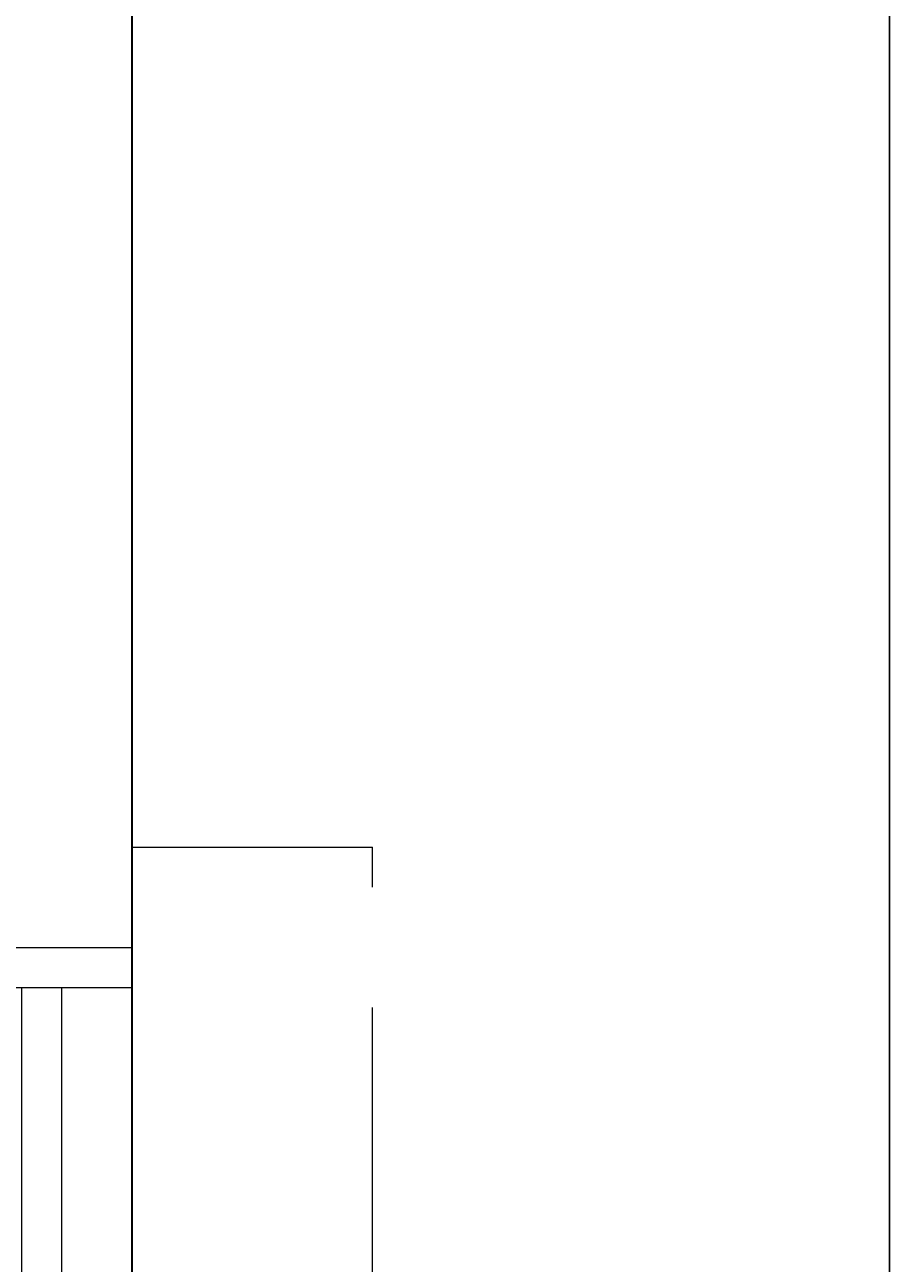
# Model space of a CAD drawing. Units: inches. Extents: x -128 to 854, y -395 to 398.
# Tile 32 of 61: x 309 to 352, y 2 to 64. Entities that reach past the tile are written whole.
import ezdxf

# ---------------------------------------------------------------- set-up
doc = ezdxf.new("R2010")
doc.units = ezdxf.units.IN
doc.header["$MEASUREMENT"] = 0
doc.linetypes.add('ACAD_ISO02W100', pattern=[15, 12, -3])
for name, color, linetype, lineweight in [('A-ANNO-DIMS', 2, 'Continuous', 18), ('A-GLAZ', 220, 'Continuous', 18), ('A-GLAZ-OVHD', 220, 'ACAD_ISO02W100', 13), ('A-WALL', 4, 'Continuous', 35)]:
    doc.layers.add(name, color=color, linetype=linetype, lineweight=lineweight)
doc.styles.get("Standard").update_dxf_attribs({"font": 'arial.ttf'})
doc.dimstyles.get("Standard").update_dxf_attribs({"dimtxt": 0.18, "dimasz": 0.18, "dimexe": 0.18, "dimexo": 0.0625, "dimgap": 0.09, "dimtad": 0, "dimtih": 1, "dimtoh": 1, "dimdec": 1, "dimzin": 0, "dimdsep": 46, "dimlunit": 4, "dimtxsty": 'Standard', "dimcen": 0.09, "dimclrd": 1, "dimclre": 2, "dimclrt": 6, "dimadec": 0, "dimazin": 0, "dimtfac": 1, "dimtdec": 1, "dimtofl": 0, "dimtmove": 0, "dimatfit": 3, "dimfxl": 1, "dimtfill": 2, "dimtfillclr": 3, "dimtolj": 1, "dimtzin": 0, "dimarcsym": 0})

# ---------------------------------------------------------------- blocks, each defined once
blk = doc.blocks.new('WIN-48IN')
for p, q in [((9, 52), (0, 52)), ((9, 50), (0, 50)), ((3.5, 50), (3.5, 2)), ((5.5, 50), (5.5, 2)), ((9, 26), (0, 26)), ((9, 2), (0, 2)), ((9, 0), (0, 0))]:
    blk.add_line(p, q)
blk = doc.blocks.new('SHADE-48IN')
at = {"ltscale": 2}
for p, q in [((12, 62), (0, 62)), ((0, 0), (0, 62)), ((12, 57), (12, 62))]:
    blk.add_line(p, q, dxfattribs=at)
blk = doc.blocks.new('*D98')
at = {"layer": 'A-ANNO-DIMS', "color": 2, "lineweight": -2, "transparency": 16777216}
for p, q in [((313.935, 348.741), (351.853, 348.741)), ((313.935, -89.259), (351.853, -89.259))]:
    blk.add_line(p, q, dxfattribs=at)
at = {"layer": 'A-ANNO-DIMS', "color": 1, "lineweight": -2, "transparency": 16777216}
for p, q in [((351.673, 348.561), (351.673, 129.923)), ((351.673, -89.079), (351.673, 129.559))]:
    blk.add_line(p, q, dxfattribs=at)
at = {"layer": 'A-ANNO-DIMS', "color": 1, "transparency": 16777216}
for points in [[(351.643, 348.561), (351.703, 348.561), (351.673, 348.741)], [(351.643, -89.079), (351.703, -89.079), (351.673, -89.259)]]:
    blk.add_solid(points, dxfattribs=at)
at = {"layer": 'Defpoints', "color": 0, "transparency": 16777216}
for p in [(313.873, 348.741), (351.673, 348.741), (313.873, -89.259)]:
    blk.add_point(p, dxfattribs=at)
at = {"layer": 'A-ANNO-DIMS', "color": 6, "transparency": 16777216, "insert": (351.673, 129.741), "char_height": 0.18, "attachment_point": 5, "bg_fill": 1, "box_fill_scale": 1.25, "bg_fill_color": 3, "bg_fill_transparency": 0}
blk.add_mtext('\\A1;36\'-6"', dxfattribs=at)

msp = doc.modelspace()

# ---------------------------------------------------------------- linework, layer by layer
at = {"layer": 'A-WALL'}
msp.add_line((313.873, 348.741), (313.873, -89.259), dxfattribs=at)

# ---------------------------------------------------------------- block references
at = {"layer": 'A-GLAZ', "rotation": 180}
msp.add_blockref('WIN-48IN', (313.873, 17.741), dxfattribs=at)
at = {"layer": 'A-GLAZ-OVHD', "extrusion": (0, 0, -1), "zscale": -1}
msp.add_blockref('SHADE-48IN', (-325.873, -39.259), dxfattribs=at)

# ---------------------------------------------------------------- dimensions: what is measured, and where the dimension line sits
at = {"layer": 'A-ANNO-DIMS'}
dim = msp.add_linear_dim(base=(351.673, 348.741), p1=(313.873, -89.259), p2=(313.873, 348.741), angle=90, dimstyle='Standard', override={"dimdec": 1, "dimlfac": 1, "dimrnd": 0, "dimzin": 1, "dimdsep": 46, "dimlunit": 4, "dimfrac": 2}, dxfattribs=at)
dim.commit()
dim.dimension.update_dxf_attribs({"geometry": '*D98', "text_midpoint": (351.673, 129.741)})

doc.saveas('drawing.dxf')
